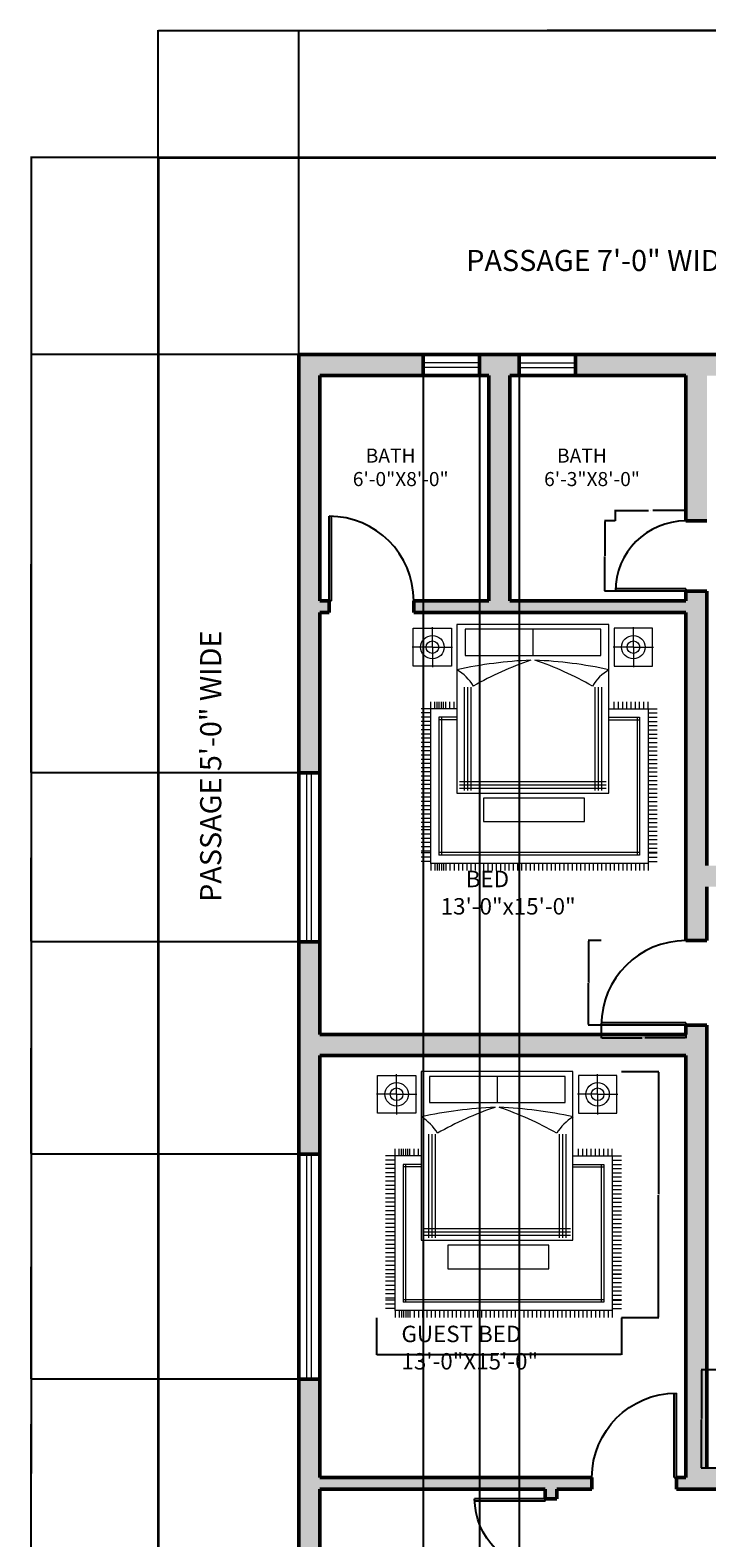
# Model space of a CAD drawing. Units: inches. Extents: x 2447 to 3157, y 2799 to 3988.
# Tile 3 of 9: x 2447 to 2735, y 3345 to 3988. Entities that reach past the tile are written whole.
import ezdxf

# ---------------------------------------------------------------- set-up
doc = ezdxf.new("R2010")
doc.units = ezdxf.units.IN
for name, color, linetype, lineweight in [('A-ANNO-DIMS', 2, 'Continuous', 18), ('A-AREA-IDEN', 7, 'Continuous', 25), ('A-DOOR', 3, 'Continuous', 25), ('A-FURN', 8, 'Continuous', 18), ('A-GLAZ', 4, 'Continuous', 18), ('A-WALL', 7, 'Continuous', 50), ('A-WALL-PATT', 252, 'Continuous', 13), ('C-PROP', 6, 'Continuous', 35)]:
    doc.layers.add(name, color=color, linetype=linetype, lineweight=lineweight)
doc.styles.get("Standard").update_dxf_attribs({"font": 'arial.ttf'})
doc.dimstyles.get("Standard").update_dxf_attribs({"dimtxt": 0.18, "dimasz": 0.18, "dimexe": 0.18, "dimexo": 0.0625, "dimgap": 0.09, "dimtad": 0, "dimtih": 1, "dimtoh": 1, "dimdec": 4, "dimzin": 0, "dimdsep": 46, "dimtxsty": 'Standard', "dimcen": 0.09, "dimadec": 0, "dimazin": 0, "dimtfac": 1, "dimtdec": 4, "dimtofl": 0, "dimtmove": 0, "dimatfit": 3, "dimfxl": 1, "dimtolj": 1, "dimtzin": 0, "dimarcsym": 0})

# ---------------------------------------------------------------- blocks, each defined once
blk = doc.blocks.new('A$C462B680F')
for p, q in [((0.011, 2.874, -0.291), (0.465, 2.874, -0.291)), ((0.011, 2.424, -0.291), (0.011, 2.874, -0.291)), ((0.238, 2.649, -0.561), (0.238, 2.887, -0.561)), ((0.465, 2.874, -0.291), (0.465, 2.424, -0.291)), ((2.33, 2.918, -0.291), (0.53, 2.918, -0.291)), ((0.53, 2.918, -0.291), (0.53, 0.918, -0.291)), ((2.33, 0.918, -0.291), (2.33, 2.918, -0.291)), ((2.849, 2.874, -0.291), (2.395, 2.874, -0.291)), ((2.395, 2.874, -0.291), (2.395, 2.424, -0.291)), ((2.622, 2.649, -0.561), (2.622, 2.887, -0.561)), ((2.849, 2.424, -0.291), (2.849, 2.874, -0.291)), ((1.434, 2.861, -0.291), (0.627, 2.861, -0.291)), ((0.627, 2.861, -0.291), (0.627, 2.55, -0.291)), ((1.43, 2.861, -0.291), (1.43, 2.55, -0.291)), ((2.237, 2.861, -0.291), (1.43, 2.861, -0.291)), ((1.434, 2.55, -0.291), (1.434, 2.861, -0.291)), ((2.237, 2.55, -0.291), (2.237, 2.861, -0.291)), ((0.238, 2.649, -0.561), (0, 2.649, -0.561)), ((0.238, 2.649, -0.561), (0.238, 2.411, -0.561)), ((0.238, 2.649, -0.561), (0.476, 2.649, -0.561)), ((0.627, 2.55, -0.291), (1.434, 2.55, -0.291)), ((1.43, 2.55, -0.291), (2.237, 2.55, -0.291)), ((2.622, 2.649, -0.561), (2.384, 2.649, -0.561)), ((2.622, 2.649, -0.561), (2.622, 2.411, -0.561)), ((2.622, 2.649, -0.561), (2.861, 2.649, -0.561)), ((0.465, 2.424, -0.291), (0.011, 2.424, -0.291)), ((2.395, 2.424, -0.291), (2.849, 2.424, -0.291)), ((0.615, 2.176, -0.291), (0.615, 0.947, -0.291)), ((0.655, 2.176, -0.291), (0.655, 0.947, -0.291)), ((0.695, 2.176, -0.291), (0.695, 0.947, -0.291)), ((2.165, 2.176, -0.291), (2.165, 0.947, -0.291)), ((2.205, 2.176, -0.291), (2.205, 0.947, -0.291)), ((2.245, 2.176, -0.291), (2.245, 0.947, -0.291)), ((0.219, 1.918, -0.291), (0.219, 2, -0.291)), ((0.269, 1.918, -0.291), (0.269, 2, -0.291)), ((0.296, 1.918, -0.291), (0.296, 2, -0.291)), ((0.319, 1.918, -0.291), (0.319, 2, -0.291)), ((0.346, 1.918, -0.291), (0.346, 2, -0.291)), ((0.369, 1.918, -0.291), (0.369, 2, -0.291)), ((0.396, 1.918, -0.291), (0.396, 2, -0.291)), ((0.446, 1.918, -0.291), (0.446, 2, -0.291)), ((0.496, 1.918, -0.291), (0.496, 2, -0.291)), ((2.396, 1.918, -0.291), (2.396, 2, -0.291)), ((2.446, 1.918, -0.291), (2.446, 2, -0.291)), ((2.496, 1.918, -0.291), (2.496, 2, -0.291)), ((2.546, 1.918, -0.291), (2.546, 2, -0.291)), ((2.596, 1.918, -0.291), (2.596, 2, -0.291)), ((2.646, 1.918, -0.291), (2.646, 2, -0.291)), ((2.696, 1.918, -0.291), (2.696, 2, -0.291)), ((2.746, 1.918, -0.291), (2.746, 2, -0.291)), ((2.796, 1.918, -0.291), (2.796, 2, -0.291)), ((0.215, 1.918, -0.291), (0.105, 1.918, -0.291)), ((0.215, 1.868, -0.291), (0.105, 1.868, -0.291)), ((0.215, 1.818, -0.291), (0.105, 1.818, -0.291)), ((0.215, 1.918, -0.291), (0.215, 0.082, -0.291)), ((0.53, 1.918, -0.291), (0.215, 1.918, -0.291)), ((0.315, 1.818, -0.291), (0.315, 0.182, -0.291)), ((0.53, 1.818, -0.291), (0.315, 1.818, -0.291)), ((0.345, 1.818, -0.291), (0.345, 0.182, -0.291)), ((2.33, 1.918, -0.291), (2.796, 1.918, -0.291)), ((2.33, 1.818, -0.291), (2.696, 1.818, -0.291)), ((2.666, 1.818, -0.291), (2.666, 0.182, -0.291)), ((2.696, 1.818, -0.291), (2.696, 0.182, -0.291)), ((2.796, 1.918, -0.291), (2.796, 0.082, -0.291)), ((2.796, 1.918, -0.291), (2.906, 1.918, -0.291)), ((2.796, 1.868, -0.291), (2.906, 1.868, -0.291)), ((2.796, 1.818, -0.291), (2.906, 1.818, -0.291)), ((0.215, 1.768, -0.291), (0.105, 1.768, -0.291)), ((0.215, 1.718, -0.291), (0.105, 1.718, -0.291)), ((0.215, 1.668, -0.291), (0.105, 1.668, -0.291)), ((0.215, 1.618, -0.291), (0.105, 1.618, -0.291)), ((0.53, 1.788, -0.291), (0.315, 1.788, -0.291)), ((2.33, 1.788, -0.291), (2.696, 1.788, -0.291)), ((2.796, 1.768, -0.291), (2.906, 1.768, -0.291)), ((2.796, 1.718, -0.291), (2.906, 1.718, -0.291)), ((2.796, 1.668, -0.291), (2.906, 1.668, -0.291)), ((2.796, 1.618, -0.291), (2.906, 1.618, -0.291)), ((0.215, 1.568, -0.291), (0.105, 1.568, -0.291)), ((0.215, 1.518, -0.291), (0.105, 1.518, -0.291)), ((0.215, 1.468, -0.291), (0.105, 1.468, -0.291)), ((2.796, 1.568, -0.291), (2.906, 1.568, -0.291)), ((2.796, 1.518, -0.291), (2.906, 1.518, -0.291)), ((2.796, 1.468, -0.291), (2.906, 1.468, -0.291)), ((0.215, 1.418, -0.291), (0.105, 1.418, -0.291)), ((0.215, 1.368, -0.291), (0.105, 1.368, -0.291)), ((0.215, 1.318, -0.291), (0.105, 1.318, -0.291)), ((0.215, 1.268, -0.291), (0.105, 1.268, -0.291)), ((2.796, 1.418, -0.291), (2.906, 1.418, -0.291)), ((2.796, 1.368, -0.291), (2.906, 1.368, -0.291)), ((2.796, 1.318, -0.291), (2.906, 1.318, -0.291)), ((2.796, 1.268, -0.291), (2.906, 1.268, -0.291)), ((0.215, 1.218, -0.291), (0.105, 1.218, -0.291)), ((0.215, 1.168, -0.291), (0.105, 1.168, -0.291)), ((0.215, 1.118, -0.291), (0.105, 1.118, -0.291)), ((2.796, 1.218, -0.291), (2.906, 1.218, -0.291)), ((2.796, 1.168, -0.291), (2.906, 1.168, -0.291)), ((2.796, 1.118, -0.291), (2.906, 1.118, -0.291)), ((0.215, 1.068, -0.291), (0.105, 1.068, -0.291)), ((0.215, 1.018, -0.291), (0.105, 1.018, -0.291)), ((0.215, 0.968, -0.291), (0.105, 0.968, -0.291)), ((0.215, 0.918, -0.291), (0.105, 0.918, -0.291)), ((0.53, 0.918, -0.291), (2.33, 0.918, -0.291)), ((0.558, 1.057, -0.291), (2.299, 1.057, -0.291)), ((0.558, 1.017, -0.291), (2.299, 1.017, -0.291)), ((0.558, 0.977, -0.291), (2.299, 0.977, -0.291)), ((2.796, 1.068, -0.291), (2.906, 1.068, -0.291)), ((2.796, 1.018, -0.291), (2.906, 1.018, -0.291)), ((2.796, 0.968, -0.291), (2.906, 0.968, -0.291)), ((2.796, 0.918, -0.291), (2.906, 0.918, -0.291)), ((0.215, 0.868, -0.291), (0.105, 0.868, -0.291)), ((0.215, 0.818, -0.291), (0.105, 0.818, -0.291)), ((0.215, 0.768, -0.291), (0.105, 0.768, -0.291)), ((0.215, 0.718, -0.291), (0.105, 0.718, -0.291)), ((0.844, 0.859, -0.291), (0.844, 0.579, -0.291)), ((2.044, 0.859, -0.291), (0.844, 0.859, -0.291)), ((2.044, 0.579, -0.291), (2.044, 0.859, -0.291)), ((2.796, 0.868, -0.291), (2.906, 0.868, -0.291)), ((2.796, 0.818, -0.291), (2.906, 0.818, -0.291)), ((2.796, 0.768, -0.291), (2.906, 0.768, -0.291)), ((2.796, 0.718, -0.291), (2.906, 0.718, -0.291)), ((0.215, 0.668, -0.291), (0.105, 0.668, -0.291)), ((0.215, 0.618, -0.291), (0.105, 0.618, -0.291)), ((0.215, 0.568, -0.291), (0.105, 0.568, -0.291)), ((0.844, 0.579, -0.291), (2.044, 0.579, -0.291)), ((2.796, 0.668, -0.291), (2.906, 0.668, -0.291)), ((2.796, 0.618, -0.291), (2.906, 0.618, -0.291)), ((2.796, 0.568, -0.291), (2.906, 0.568, -0.291)), ((0.215, 0.518, -0.291), (0.105, 0.518, -0.291)), ((0.215, 0.48, -0.291), (0.105, 0.48, -0.291)), ((0.215, 0.43, -0.291), (0.105, 0.43, -0.291)), ((0.215, 0.38, -0.291), (0.105, 0.38, -0.291)), ((2.796, 0.518, -0.291), (2.906, 0.518, -0.291)), ((2.796, 0.516, -0.291), (2.906, 0.516, -0.291)), ((2.796, 0.466, -0.291), (2.906, 0.466, -0.291)), ((2.796, 0.416, -0.291), (2.906, 0.416, -0.291)), ((2.796, 0.366, -0.291), (2.906, 0.366, -0.291)), ((0.215, 0.33, -0.291), (0.105, 0.33, -0.291)), ((0.215, 0.28, -0.291), (0.105, 0.28, -0.291)), ((0.215, 0.23, -0.291), (0.105, 0.23, -0.291)), ((0.215, 0.207, -0.291), (0.105, 0.207, -0.291)), ((0.215, 0.207, -0.291), (0.105, 0.207, -0.291)), ((2.696, 0.212, -0.291), (0.315, 0.212, -0.291)), ((2.696, 0.182, -0.291), (0.315, 0.182, -0.291)), ((2.796, 0.316, -0.291), (2.906, 0.316, -0.291)), ((2.796, 0.266, -0.291), (2.906, 0.266, -0.291)), ((2.796, 0.216, -0.291), (2.906, 0.216, -0.291)), ((2.796, 0.207, -0.291), (2.906, 0.207, -0.291)), ((2.796, 0.207, -0.291), (2.906, 0.207, -0.291)), ((0.215, 0.157, -0.291), (0.105, 0.157, -0.291)), ((0.215, 0.107, -0.291), (0.105, 0.107, -0.291)), ((2.796, 0.082, -0.291), (0.215, 0.082, -0.291)), ((0.219, 0.082, -0.291), (0.219, 0, -0.291)), ((0.269, 0.082, -0.291), (0.269, 0, -0.291)), ((0.296, 0.082, -0.291), (0.296, 0, -0.291)), ((0.319, 0.082, -0.291), (0.319, 0, -0.291)), ((0.346, 0.082, -0.291), (0.346, 0, -0.291)), ((0.369, 0.082, -0.291), (0.369, 0, -0.291)), ((0.396, 0.082, -0.291), (0.396, 0, -0.291)), ((0.446, 0.082, -0.291), (0.446, 0, -0.291)), ((0.496, 0.082, -0.291), (0.496, 0, -0.291)), ((0.546, 0.082, -0.291), (0.546, 0, -0.291)), ((0.596, 0.082, -0.291), (0.596, 0, -0.291)), ((0.646, 0.082, -0.291), (0.646, 0, -0.291)), ((0.696, 0.082, -0.291), (0.696, 0, -0.291)), ((0.746, 0.082, -0.291), (0.746, 0, -0.291)), ((0.796, 0.082, -0.291), (0.796, 0, -0.291)), ((0.846, 0.082, -0.291), (0.846, 0, -0.291)), ((0.896, 0.082, -0.291), (0.896, 0, -0.291)), ((0.946, 0.082, -0.291), (0.946, 0, -0.291)), ((0.996, 0.082, -0.291), (0.996, 0, -0.291)), ((1.046, 0.082, -0.291), (1.046, 0, -0.291)), ((1.096, 0.082, -0.291), (1.096, 0, -0.291)), ((1.146, 0.082, -0.291), (1.146, 0, -0.291)), ((1.196, 0.082, -0.291), (1.196, 0, -0.291)), ((1.246, 0.082, -0.291), (1.246, 0, -0.291)), ((1.296, 0.082, -0.291), (1.296, 0, -0.291)), ((1.346, 0.082, -0.291), (1.346, 0, -0.291)), ((1.346, 0.082, -0.291), (1.346, 0, -0.291)), ((1.396, 0.082, -0.291), (1.396, 0, -0.291)), ((1.396, 0.082, -0.291), (1.396, 0, -0.291)), ((1.446, 0.082, -0.291), (1.446, 0, -0.291)), ((1.446, 0.082, -0.291), (1.446, 0, -0.291)), ((1.496, 0.082, -0.291), (1.496, 0, -0.291)), ((1.496, 0.082, -0.291), (1.496, 0, -0.291)), ((1.546, 0.082, -0.291), (1.546, 0, -0.291)), ((1.596, 0.082, -0.291), (1.596, 0, -0.291)), ((1.646, 0.082, -0.291), (1.646, 0, -0.291)), ((1.696, 0.082, -0.291), (1.696, 0, -0.291)), ((1.746, 0.082, -0.291), (1.746, 0, -0.291)), ((1.796, 0.082, -0.291), (1.796, 0, -0.291)), ((1.846, 0.082, -0.291), (1.846, 0, -0.291)), ((1.846, 0.082, -0.291), (1.846, 0, -0.291)), ((1.896, 0.082, -0.291), (1.896, 0, -0.291)), ((1.946, 0.082, -0.291), (1.946, 0, -0.291)), ((1.996, 0.082, -0.291), (1.996, 0, -0.291)), ((2.046, 0.082, -0.291), (2.046, 0, -0.291)), ((2.096, 0.082, -0.291), (2.096, 0, -0.291)), ((2.146, 0.082, -0.291), (2.146, 0, -0.291)), ((2.196, 0.082, -0.291), (2.196, 0, -0.291)), ((2.246, 0.082, -0.291), (2.246, 0, -0.291)), ((2.296, 0.082, -0.291), (2.296, 0, -0.291)), ((2.346, 0.082, -0.291), (2.346, 0, -0.291)), ((2.396, 0.082, -0.291), (2.396, 0, -0.291)), ((2.446, 0.082, -0.291), (2.446, 0, -0.291)), ((2.496, 0.082, -0.291), (2.496, 0, -0.291)), ((2.546, 0.082, -0.291), (2.546, 0, -0.291)), ((2.596, 0.082, -0.291), (2.596, 0, -0.291)), ((2.646, 0.082, -0.291), (2.646, 0, -0.291)), ((2.696, 0.082, -0.291), (2.696, 0, -0.291)), ((2.746, 0.082, -0.291), (2.746, 0, -0.291)), ((2.796, 0.157, -0.291), (2.906, 0.157, -0.291)), ((2.796, 0.107, -0.291), (2.906, 0.107, -0.291)), ((2.796, 0.082, -0.291), (2.796, 0, -0.291))]:
    blk.add_line(p, q)
for centre, radius in [((0.238, 2.649, -0.561), 0.139), ((0.238, 2.649, -0.561), 0.075), ((2.622, 2.649, -0.561), 0.139), ((2.622, 2.649, -0.561), 0.075)]:
    blk.add_circle(centre, radius)
for centre, radius, start, end in [((1.618, -2.572, -0.291), 5.071, 92.3872, 102.3913), ((0.231, 1.886, -0.291), 0.578, 31.4118, 58.8491), ((2.601, -1.074, -0.291), 3.763, 108.5127, 119.9306), ((1.243, -2.572, -0.291), 5.071, 77.6087, 87.6128), ((0.259, -1.074, -0.291), 3.763, 60.0694, 71.4873), ((2.63, 1.886, -0.291), 0.578, 121.1509, 148.5882)]:
    blk.add_arc(centre, radius, start, end)
blk = doc.blocks.new('DOOR-SWING-36IN')
for p, q in [((0, 0), (0, 36)), ((1, 0), (1, 35.99)), ((1, 0), (0, 0))]:
    blk.add_line(p, q)
blk.add_arc((0, 0), 36, 0, 90)
blk = doc.blocks.new('DOOR-SWING-30IN')
for p, q in [((0, 1), (-29.98, 1)), ((0, 1), (0, 0)), ((0, 0), (-30, 0))]:
    blk.add_line(p, q)
blk.add_arc((0, 0), 30, 90, 180)
blk = doc.blocks.new('GLAZING-24IN')
for p, q in [((0, 0), (0, 24)), ((2, 0), (2, 24))]:
    blk.add_line(p, q)
blk = doc.blocks.new('*D16')
at = {"layer": 'A-ANNO-DIMS', "color": 0, "lineweight": -2, "transparency": 16777216}
for p, q in [((2690.3, 3599.7), (2684.79, 3599.7)), ((2684.97, 3599.52), (2684.97, 3581.88)), ((2684.97, 3563.88), (2684.97, 3581.52)), ((2690.3, 3563.7), (2684.79, 3563.7))]:
    blk.add_line(p, q, dxfattribs=at)
at = {"layer": 'A-ANNO-DIMS', "color": 0, "transparency": 16777216}
for points in [[(2684.94, 3599.52), (2685, 3599.52), (2684.97, 3599.7)], [(2684.94, 3563.88), (2685, 3563.88), (2684.97, 3563.7)]]:
    blk.add_solid(points, dxfattribs=at)
at = {"layer": 'Defpoints', "color": 0, "transparency": 16777216}
for p in [(2684.97, 3599.7), (2690.37, 3599.7), (2690.37, 3563.7)]:
    blk.add_point(p, dxfattribs=at)
at = {"layer": 'A-ANNO-DIMS', "color": 0, "transparency": 16777216, "insert": (2684.97, 3581.7), "char_height": 0.18, "attachment_point": 5}
blk.add_mtext('\\A1;DOOR 36 TYP.', dxfattribs=at)
blk = doc.blocks.new('*D17')
at = {"layer": 'A-ANNO-DIMS', "color": 0, "lineweight": -2, "transparency": 16777216}
for p, q in [((2690.37, 3563.64), (2690.37, 3558.12)), ((2726.37, 3563.64), (2726.37, 3558.12)), ((2690.55, 3558.3), (2707.84, 3558.3)), ((2726.19, 3558.3), (2708.9, 3558.3))]:
    blk.add_line(p, q, dxfattribs=at)
at = {"layer": 'A-ANNO-DIMS', "color": 0, "transparency": 16777216}
for points in [[(2690.55, 3558.33), (2690.55, 3558.27), (2690.37, 3558.3)], [(2726.19, 3558.33), (2726.19, 3558.27), (2726.37, 3558.3)]]:
    blk.add_solid(points, dxfattribs=at)
at = {"layer": 'Defpoints', "color": 0, "transparency": 16777216}
for p in [(2690.37, 3563.7), (2726.37, 3563.7), (2690.37, 3558.3)]:
    blk.add_point(p, dxfattribs=at)
at = {"layer": 'A-ANNO-DIMS', "color": 0, "transparency": 16777216, "insert": (2708.37, 3558.3), "char_height": 0.18, "attachment_point": 5}
blk.add_mtext('\\A1;36 TYP.', dxfattribs=at)
blk = doc.blocks.new('*D18')
at = {"layer": 'A-ANNO-DIMS', "color": 0, "lineweight": -2, "transparency": 16777216}
for p, q in [((2696.37, 3778.76), (2696.37, 3783.38)), ((2696.55, 3783.2), (2710.43, 3783.2)), ((2726.19, 3783.2), (2712.3, 3783.2)), ((2726.37, 3778.76), (2726.37, 3783.38))]:
    blk.add_line(p, q, dxfattribs=at)
at = {"layer": 'A-ANNO-DIMS', "color": 0, "transparency": 16777216}
for points in [[(2696.55, 3783.23), (2696.55, 3783.17), (2696.37, 3783.2)], [(2726.19, 3783.23), (2726.19, 3783.17), (2726.37, 3783.2)]]:
    blk.add_solid(points, dxfattribs=at)
at = {"layer": 'Defpoints', "color": 0, "transparency": 16777216}
for p in [(2726.37, 3783.2), (2696.37, 3778.7), (2726.37, 3778.7)]:
    blk.add_point(p, dxfattribs=at)
at = {"layer": 'A-ANNO-DIMS', "color": 0, "transparency": 16777216, "insert": (2711.37, 3783.2), "char_height": 0.18, "attachment_point": 5}
blk.add_mtext('\\A1;DOOR 30 TYP.', dxfattribs=at)
blk = doc.blocks.new('*D19')
at = {"layer": 'A-ANNO-DIMS', "color": 0, "lineweight": -2, "transparency": 16777216}
for p, q in [((2696.3, 3778.7), (2691.69, 3778.7)), ((2691.87, 3778.52), (2691.87, 3763.88)), ((2691.87, 3748.88), (2691.87, 3763.52)), ((2696.3, 3748.7), (2691.69, 3748.7))]:
    blk.add_line(p, q, dxfattribs=at)
at = {"layer": 'A-ANNO-DIMS', "color": 0, "transparency": 16777216}
for points in [[(2691.84, 3778.52), (2691.9, 3778.52), (2691.87, 3778.7)], [(2691.84, 3748.88), (2691.9, 3748.88), (2691.87, 3748.7)]]:
    blk.add_solid(points, dxfattribs=at)
at = {"layer": 'Defpoints', "color": 0, "transparency": 16777216}
for p in [(2691.87, 3778.7), (2696.37, 3778.7), (2696.37, 3748.7)]:
    blk.add_point(p, dxfattribs=at)
at = {"layer": 'A-ANNO-DIMS', "color": 0, "transparency": 16777216, "insert": (2691.87, 3763.7), "char_height": 0.18, "attachment_point": 5}
blk.add_mtext('\\A1;30 TYP.', dxfattribs=at)
blk = doc.blocks.new('*D20')
at = {"layer": 'A-ANNO-DIMS', "color": 0, "lineweight": -2, "transparency": 16777216}
for p, q in [((2739.3, 3416.7), (2732.89, 3416.7)), ((2733.07, 3416.52), (2733.07, 3395.88)), ((2733.07, 3374.88), (2733.07, 3395.52)), ((2739.3, 3374.7), (2732.89, 3374.7))]:
    blk.add_line(p, q, dxfattribs=at)
at = {"layer": 'A-ANNO-DIMS', "color": 0, "transparency": 16777216}
for points in [[(2733.04, 3416.52), (2733.1, 3416.52), (2733.07, 3416.7)], [(2733.04, 3374.88), (2733.1, 3374.88), (2733.07, 3374.7)]]:
    blk.add_solid(points, dxfattribs=at)
at = {"layer": 'Defpoints', "color": 0, "transparency": 16777216}
for p in [(2733.07, 3416.7), (2739.37, 3416.7), (2739.37, 3374.7)]:
    blk.add_point(p, dxfattribs=at)
at = {"layer": 'A-ANNO-DIMS', "color": 0, "transparency": 16777216, "insert": (2733.07, 3395.7), "char_height": 0.18, "attachment_point": 5}
blk.add_mtext('\\A1;DOOR 42 TYP.', dxfattribs=at)
blk = doc.blocks.new('*D26')
at = {"layer": 'A-ANNO-DIMS', "color": 0, "lineweight": -2, "transparency": 16777216}
for p, q in [((2699.05, 3543.84), (2714.9, 3543.84)), ((2714.72, 3543.66), (2714.72, 3491.58)), ((2714.72, 3439.13), (2714.72, 3491.21)), ((2699.05, 3438.95), (2714.9, 3438.95))]:
    blk.add_line(p, q, dxfattribs=at)
at = {"layer": 'A-ANNO-DIMS', "color": 0, "transparency": 16777216}
for points in [[(2714.69, 3543.66), (2714.75, 3543.66), (2714.72, 3543.84)], [(2714.69, 3439.13), (2714.75, 3439.13), (2714.72, 3438.95)]]:
    blk.add_solid(points, dxfattribs=at)
at = {"layer": 'Defpoints', "color": 0, "transparency": 16777216}
for p in [(2698.99, 3543.84), (2714.72, 3543.84), (2698.99, 3438.95)]:
    blk.add_point(p, dxfattribs=at)
at = {"layer": 'A-ANNO-DIMS', "color": 0, "transparency": 16777216, "insert": (2714.72, 3491.39), "char_height": 0.18, "attachment_point": 5}
blk.add_mtext('\\A1;BED GROUP 105 TYP.', dxfattribs=at)
blk = doc.blocks.new('*D27')
at = {"layer": 'A-ANNO-DIMS', "color": 0, "lineweight": -2, "transparency": 16777216}
for p, q in [((2594.54, 3438.88), (2594.54, 3423.03)), ((2698.99, 3438.88), (2698.99, 3423.03)), ((2594.72, 3423.21), (2646.18, 3423.21)), ((2698.81, 3423.21), (2647.36, 3423.21))]:
    blk.add_line(p, q, dxfattribs=at)
at = {"layer": 'A-ANNO-DIMS', "color": 0, "transparency": 16777216}
for points in [[(2594.72, 3423.24), (2594.72, 3423.18), (2594.54, 3423.21)], [(2698.81, 3423.24), (2698.81, 3423.18), (2698.99, 3423.21)]]:
    blk.add_solid(points, dxfattribs=at)
at = {"layer": 'Defpoints', "color": 0, "transparency": 16777216}
for p in [(2594.54, 3438.95), (2698.99, 3438.95), (2698.99, 3423.21)]:
    blk.add_point(p, dxfattribs=at)
at = {"layer": 'A-ANNO-DIMS', "color": 0, "transparency": 16777216, "insert": (2646.77, 3423.21), "char_height": 0.18, "attachment_point": 5}
blk.add_mtext('\\A1;104 TYP.', dxfattribs=at)
blk = doc.blocks.new('*D45')
at = {"layer": 'A-ANNO-DIMS', "color": 0, "lineweight": -2, "transparency": 16777216}
for p, q in [((2501.3, 3933.7), (2447.04, 3933.7)), ((2447.22, 3933.52), (2447.22, 3393.88)), ((2447.22, 2853.88), (2447.22, 3393.52)), ((2501.3, 2853.7), (2447.04, 2853.7))]:
    blk.add_line(p, q, dxfattribs=at)
at = {"layer": 'A-ANNO-DIMS', "color": 0, "transparency": 16777216}
for points in [[(2447.19, 3933.52), (2447.25, 3933.52), (2447.22, 3933.7)], [(2447.19, 2853.88), (2447.25, 2853.88), (2447.22, 2853.7)]]:
    blk.add_solid(points, dxfattribs=at)
at = {"layer": 'Defpoints', "color": 0, "transparency": 16777216}
for p in [(2447.22, 3933.7), (2501.37, 3933.7), (2501.37, 2853.7)]:
    blk.add_point(p, dxfattribs=at)
at = {"layer": 'A-ANNO-DIMS', "color": 0, "transparency": 16777216, "insert": (2447.22, 3393.7), "char_height": 0.18, "attachment_point": 5}
blk.add_mtext('\\A1;1080', dxfattribs=at)
blk = doc.blocks.new('*D46')
at = {"layer": 'A-ANNO-DIMS', "color": 0, "lineweight": -2, "transparency": 16777216}
for p, q in [((2561.37, 3849.76), (2561.37, 3988.03)), ((2561.55, 3987.85), (2803.57, 3987.85)), ((3046.19, 3987.85), (2804.16, 3987.85)), ((3046.37, 3825.76), (3046.37, 3988.03))]:
    blk.add_line(p, q, dxfattribs=at)
at = {"layer": 'A-ANNO-DIMS', "color": 0, "transparency": 16777216}
for points in [[(2561.55, 3987.88), (2561.55, 3987.82), (2561.37, 3987.85)], [(3046.19, 3987.88), (3046.19, 3987.82), (3046.37, 3987.85)]]:
    blk.add_solid(points, dxfattribs=at)
at = {"layer": 'Defpoints', "color": 0, "transparency": 16777216}
for p in [(3046.37, 3987.85), (2561.37, 3849.7), (3046.37, 3825.7)]:
    blk.add_point(p, dxfattribs=at)
at = {"layer": 'A-ANNO-DIMS', "color": 0, "transparency": 16777216, "insert": (2803.87, 3987.85), "char_height": 0.18, "attachment_point": 5}
blk.add_mtext('\\A1;485', dxfattribs=at)
blk = doc.blocks.new('*D52')
at = {"layer": 'A-ANNO-DIMS', "color": 0, "lineweight": -2, "transparency": 16777216}
for p, q in [((2501.37, 3933.76), (2501.37, 3988.03)), ((2501.55, 3987.85), (2666.54, 3987.85)), ((2832.28, 3987.85), (2667.29, 3987.85)), ((2832.46, 3933.76), (2832.46, 3988.03))]:
    blk.add_line(p, q, dxfattribs=at)
at = {"layer": 'A-ANNO-DIMS', "color": 0, "transparency": 16777216}
for points in [[(2501.55, 3987.88), (2501.55, 3987.82), (2501.37, 3987.85)], [(2832.28, 3987.88), (2832.28, 3987.82), (2832.46, 3987.85)]]:
    blk.add_solid(points, dxfattribs=at)
at = {"layer": 'Defpoints', "color": 0, "transparency": 16777216}
for p in [(2832.46, 3987.85), (2501.37, 3933.7), (2832.46, 3933.7)]:
    blk.add_point(p, dxfattribs=at)
at = {"layer": 'A-ANNO-DIMS', "color": 0, "transparency": 16777216, "insert": (2666.91, 3987.85), "char_height": 0.18, "attachment_point": 5}
blk.add_mtext('\\A1;331.1', dxfattribs=at)
blk = doc.blocks.new('*D57')
at = {"layer": 'A-ANNO-DIMS', "color": 0, "lineweight": -2, "transparency": 16777216}
for p, q in [((2561.3, 3412.7), (2447.04, 3412.7)), ((2447.22, 3412.52), (2447.22, 3372.5)), ((2447.22, 3332.11), (2447.22, 3372.13)), ((2561.3, 3331.93), (2447.04, 3331.93))]:
    blk.add_line(p, q, dxfattribs=at)
at = {"layer": 'A-ANNO-DIMS', "color": 0, "transparency": 16777216}
for points in [[(2447.19, 3412.52), (2447.25, 3412.52), (2447.22, 3412.7)], [(2447.19, 3332.11), (2447.25, 3332.11), (2447.22, 3331.93)]]:
    blk.add_solid(points, dxfattribs=at)
at = {"layer": 'Defpoints', "color": 0, "transparency": 16777216}
for p in [(2447.22, 3412.7), (2561.37, 3412.7), (2561.37, 3331.93)]:
    blk.add_point(p, dxfattribs=at)
at = {"layer": 'A-ANNO-DIMS', "color": 0, "transparency": 16777216, "insert": (2447.22, 3372.31), "char_height": 0.18, "attachment_point": 5}
blk.add_mtext('\\A1;80.77', dxfattribs=at)
blk = doc.blocks.new('*D58')
at = {"layer": 'A-ANNO-DIMS', "color": 0, "lineweight": -2, "transparency": 16777216}
for p, q in [((2561.3, 3508.7), (2447.04, 3508.7)), ((2447.22, 3508.52), (2447.22, 3460.88)), ((2447.22, 3412.88), (2447.22, 3460.52)), ((2561.3, 3412.7), (2447.04, 3412.7))]:
    blk.add_line(p, q, dxfattribs=at)
at = {"layer": 'A-ANNO-DIMS', "color": 0, "transparency": 16777216}
for points in [[(2447.19, 3508.52), (2447.25, 3508.52), (2447.22, 3508.7)], [(2447.19, 3412.88), (2447.25, 3412.88), (2447.22, 3412.7)]]:
    blk.add_solid(points, dxfattribs=at)
at = {"layer": 'Defpoints', "color": 0, "transparency": 16777216}
for p in [(2447.22, 3508.7), (2561.37, 3508.7), (2561.37, 3412.7)]:
    blk.add_point(p, dxfattribs=at)
at = {"layer": 'A-ANNO-DIMS', "color": 0, "transparency": 16777216, "insert": (2447.22, 3460.7), "char_height": 0.18, "attachment_point": 5}
blk.add_mtext('\\A1;96', dxfattribs=at)
blk = doc.blocks.new('*D59')
at = {"layer": 'A-ANNO-DIMS', "color": 0, "lineweight": -2, "transparency": 16777216}
for p, q in [((2561.3, 3599.25), (2447.04, 3599.25)), ((2447.22, 3599.07), (2447.22, 3554.16)), ((2447.22, 3508.88), (2447.22, 3553.79)), ((2561.3, 3508.7), (2447.04, 3508.7))]:
    blk.add_line(p, q, dxfattribs=at)
at = {"layer": 'A-ANNO-DIMS', "color": 0, "transparency": 16777216}
for points in [[(2447.19, 3599.07), (2447.25, 3599.07), (2447.22, 3599.25)], [(2447.19, 3508.88), (2447.25, 3508.88), (2447.22, 3508.7)]]:
    blk.add_solid(points, dxfattribs=at)
at = {"layer": 'Defpoints', "color": 0, "transparency": 16777216}
for p in [(2447.22, 3599.25), (2561.37, 3599.25), (2561.37, 3508.7)]:
    blk.add_point(p, dxfattribs=at)
at = {"layer": 'A-ANNO-DIMS', "color": 0, "transparency": 16777216, "insert": (2447.22, 3553.97), "char_height": 0.18, "attachment_point": 5}
blk.add_mtext('\\A1;90.55', dxfattribs=at)
blk = doc.blocks.new('*D60')
at = {"layer": 'A-ANNO-DIMS', "color": 0, "lineweight": -2, "transparency": 16777216}
for p, q in [((2561.3, 3671.25), (2447.04, 3671.25)), ((2447.22, 3671.07), (2447.22, 3635.43)), ((2447.22, 3599.43), (2447.22, 3635.07)), ((2561.3, 3599.25), (2447.04, 3599.25))]:
    blk.add_line(p, q, dxfattribs=at)
at = {"layer": 'A-ANNO-DIMS', "color": 0, "transparency": 16777216}
for points in [[(2447.19, 3671.07), (2447.25, 3671.07), (2447.22, 3671.25)], [(2447.19, 3599.43), (2447.25, 3599.43), (2447.22, 3599.25)]]:
    blk.add_solid(points, dxfattribs=at)
at = {"layer": 'Defpoints', "color": 0, "transparency": 16777216}
for p in [(2447.22, 3671.25), (2561.37, 3671.25), (2561.37, 3599.25)]:
    blk.add_point(p, dxfattribs=at)
at = {"layer": 'A-ANNO-DIMS', "color": 0, "transparency": 16777216, "insert": (2447.22, 3635.25), "char_height": 0.18, "attachment_point": 5}
blk.add_mtext('\\A1;72', dxfattribs=at)
blk = doc.blocks.new('*D61')
at = {"layer": 'A-ANNO-DIMS', "color": 0, "lineweight": -2, "transparency": 16777216}
for p, q in [((2561.3, 3849.7), (2447.04, 3849.7)), ((2447.22, 3849.52), (2447.22, 3760.66)), ((2447.22, 3671.43), (2447.22, 3760.29)), ((2561.3, 3671.25), (2447.04, 3671.25))]:
    blk.add_line(p, q, dxfattribs=at)
at = {"layer": 'A-ANNO-DIMS', "color": 0, "transparency": 16777216}
for points in [[(2447.19, 3849.52), (2447.25, 3849.52), (2447.22, 3849.7)], [(2447.19, 3671.43), (2447.25, 3671.43), (2447.22, 3671.25)]]:
    blk.add_solid(points, dxfattribs=at)
at = {"layer": 'Defpoints', "color": 0, "transparency": 16777216}
for p in [(2447.22, 3849.7), (2561.37, 3849.7), (2561.37, 3671.25)]:
    blk.add_point(p, dxfattribs=at)
at = {"layer": 'A-ANNO-DIMS', "color": 0, "transparency": 16777216, "insert": (2447.22, 3760.47), "char_height": 0.18, "attachment_point": 5}
blk.add_mtext('\\A1;178.45', dxfattribs=at)
blk = doc.blocks.new('*D68')
at = {"layer": 'A-ANNO-DIMS', "color": 0, "lineweight": -2, "transparency": 16777216}
for p, q in [((2561.37, 3849.64), (2561.37, 2799.37)), ((2614.37, 3840.64), (2614.37, 2799.37)), ((2561.55, 2799.55), (2587.65, 2799.55)), ((2614.19, 2799.55), (2588.09, 2799.55))]:
    blk.add_line(p, q, dxfattribs=at)
at = {"layer": 'A-ANNO-DIMS', "color": 0, "transparency": 16777216}
for points in [[(2561.55, 2799.58), (2561.55, 2799.52), (2561.37, 2799.55)], [(2614.19, 2799.58), (2614.19, 2799.52), (2614.37, 2799.55)]]:
    blk.add_solid(points, dxfattribs=at)
at = {"layer": 'Defpoints', "color": 0, "transparency": 16777216}
for p in [(2561.37, 3849.7), (2614.37, 3840.7), (2614.37, 2799.55)]:
    blk.add_point(p, dxfattribs=at)
at = {"layer": 'A-ANNO-DIMS', "color": 0, "transparency": 16777216, "insert": (2587.87, 2799.55), "char_height": 0.18, "attachment_point": 5}
blk.add_mtext('\\A1;53', dxfattribs=at)
blk = doc.blocks.new('*D69')
at = {"layer": 'A-ANNO-DIMS', "color": 0, "lineweight": -2, "transparency": 16777216}
for p, q in [((2638.37, 3840.64), (2638.37, 2799.37)), ((2655.37, 3840.64), (2655.37, 2799.37)), ((2638.55, 2799.55), (2646.66, 2799.55)), ((2655.19, 2799.55), (2647.08, 2799.55))]:
    blk.add_line(p, q, dxfattribs=at)
at = {"layer": 'A-ANNO-DIMS', "color": 0, "transparency": 16777216}
for points in [[(2638.55, 2799.58), (2638.55, 2799.52), (2638.37, 2799.55)], [(2655.19, 2799.58), (2655.19, 2799.52), (2655.37, 2799.55)]]:
    blk.add_solid(points, dxfattribs=at)
at = {"layer": 'Defpoints', "color": 0, "transparency": 16777216}
for p in [(2638.37, 3840.7), (2655.37, 3840.7), (2655.37, 2799.55)]:
    blk.add_point(p, dxfattribs=at)
at = {"layer": 'A-ANNO-DIMS', "color": 0, "transparency": 16777216, "insert": (2646.87, 2799.55), "char_height": 0.18, "attachment_point": 5}
blk.add_mtext('\\A1;17', dxfattribs=at)

msp = doc.modelspace()

# ---------------------------------------------------------------- hatches: boundary and pattern name
at = {"layer": 'A-WALL-PATT'}
h = msp.add_hatch(color=256, dxfattribs=at)
h.dxf.hatch_style = 1
h.paths.add_polyline_path([(2570.3672, 3550.7002), (2726.3672, 3550.7002), (2726.3672, 3370.7002), (2722.3672, 3370.7002), (2722.3672, 3365.7002), (2739.3672, 3365.7002), (2739.3672, 3374.7002), (2735.3672, 3374.7002), (2735.3672, 3563.7002), (2726.3672, 3563.7002), (2726.3672, 3559.7002), (2570.3672, 3559.7002), (2570.3672, 3599.2479), (2561.3672, 3599.2479), (2561.3672, 3508.7002), (2570.3672, 3508.7002)])
h.paths.add_polyline_path([(2570.3672, 3412.7002), (2561.3672, 3412.7002), (2561.3672, 3331.9279), (2570.3672, 3331.9279), (2570.3672, 3365.7002), (2666.3672, 3365.7002), (2666.3672, 3361.7002), (2671.3672, 3361.7002), (2671.3672, 3365.7002), (2686.3672, 3365.7002), (2686.3672, 3370.7002), (2570.3672, 3370.7002)])
h.paths.add_polyline_path([(2965.3672, 3430.7002), (2961.3672, 3430.7002), (2961.3672, 3434.7002), (2952.3672, 3434.7002), (2952.3672, 3430.7002), (2847.6393, 3430.7002), (2812.3672, 3395.4282), (2812.3672, 3374.7002), (2781.3672, 3374.7002), (2781.3672, 3365.7002), (2812.3672, 3365.7002), (2812.3672, 3347.7002), (2821.3672, 3347.7002), (2821.3672, 3391.7002), (2851.3672, 3421.7002), (2965.3672, 3421.7002)])
h.paths.add_polyline_path([(3046.3672, 3430.7002), (3033.3672, 3430.7002), (3033.3672, 3421.7002), (3037.3672, 3421.7002), (3037.3672, 3133.7002), (2971.1661, 3133.7002), (2971.1661, 3124.7002), (3046.3672, 3124.7002)])
h.paths.add_polyline_path([(3046.3672, 3825.7002), (3005.5801, 3825.7002), (3005.5801, 3816.7002), (3037.3672, 3816.7002), (3037.3672, 3655.7002), (2940.3672, 3655.7002), (2940.3672, 3646.7002), (3037.3672, 3646.7002), (3037.3672, 3514.7002), (3033.3672, 3514.7002), (3033.3672, 3505.7002), (3046.3672, 3505.7002)])
h.paths.add_polyline_path([(2821.3672, 3258.7002), (2812.3672, 3258.7002), (2812.3672, 3240.7002), (2808.3672, 3240.7002), (2808.3672, 3231.7002), (2812.3672, 3231.7002), (2812.3672, 3223.0688), (2821.3672, 3223.0688)])
h.paths.add_polyline_path([(2766.3672, 3240.7002), (2707.3672, 3240.7002), (2707.3672, 3234.4466, -1), (2570.3672, 3234.4466), (2570.3672, 3240.5271), (2561.3672, 3240.5271), (2561.3672, 3234.4466, 0.98243292), (2716.3185, 3231.7002), (2766.3672, 3231.7002)])
h.paths.add_polyline_path([(2570.3672, 3307.9279), (2561.3672, 3307.9279), (2561.3672, 3281.7773), (2570.3672, 3281.7773), (2570.3672, 3284.7002), (2671.3672, 3284.7002), (2671.3672, 3331.7002), (2666.3672, 3331.7002), (2666.3672, 3293.7002), (2570.3672, 3293.7002)])
h.paths.add_polyline_path([(2570.3672, 3739.7002), (2574.3672, 3739.7002), (2574.3672, 3744.7002), (2570.3672, 3744.7002), (2570.3672, 3840.7002), (2614.3672, 3840.7002), (2614.3672, 3849.7002), (2561.3672, 3849.7002), (2561.3672, 3671.2479), (2570.3672, 3671.2479)])
h.paths.add_polyline_path([(2735.3672, 3840.7002), (2789.3672, 3840.7002), (2789.3672, 3816.7002), (2798.3672, 3816.7002), (2798.3672, 3849.7002), (2679.3672, 3849.7002), (2679.3672, 3840.7002), (2726.3672, 3840.7002), (2726.3672, 3778.7002), (2735.3672, 3778.7002)])
h.paths.add_polyline_path([(2651.3672, 3840.7002), (2655.3672, 3840.7002), (2655.3672, 3849.7002), (2638.3672, 3849.7002), (2638.3672, 3840.7002), (2642.3672, 3840.7002), (2642.3672, 3744.7002), (2610.3672, 3744.7002), (2610.3672, 3739.7002), (2726.3672, 3739.7002), (2726.3672, 3599.7002), (2735.3672, 3599.7002), (2735.3672, 3622.7002), (2739.3672, 3622.7002), (2739.3672, 3631.7002), (2735.3672, 3631.7002), (2735.3672, 3748.7002), (2726.3672, 3748.7002), (2726.3672, 3744.7002), (2651.3672, 3744.7002)])
h.paths.add_polyline_path([(2900.3672, 3816.7002), (2904.3672, 3816.7002), (2904.3672, 3825.7002), (2882.3672, 3825.7002), (2882.3672, 3816.7002), (2891.3672, 3816.7002), (2891.3672, 3650.4282), (2872.6393, 3631.7002), (2775.3672, 3631.7002), (2775.3672, 3622.7002), (2876.3672, 3622.7002), (2900.3672, 3646.7002), (2904.3672, 3646.7002), (2904.3672, 3655.7002), (2900.3672, 3655.7002)])
h.paths.add_polyline_path([(2957.5801, 3825.7002), (2940.3672, 3825.7002), (2940.3672, 3816.7002), (2957.5801, 3816.7002)], flags=17)

# ---------------------------------------------------------------- linework, layer by layer
at = {"layer": 'A-GLAZ'}
for p, q in [((2564.8672, 3599.2479), (2564.8672, 3671.2479)), ((2566.8672, 3599.2479), (2566.8672, 3671.2479)), ((2564.8672, 3412.7002), (2564.8672, 3508.7002)), ((2566.8672, 3412.7002), (2566.8672, 3508.7002))]:
    msp.add_line(p, q, dxfattribs=at)
at = {"layer": 'A-WALL'}
for p, q in [((2561.3672, 3849.7002), (2561.3672, 3234.4466)), ((2561.3672, 3849.7002), (2798.3672, 3849.7002)), ((2614.3672, 3849.7002), (2614.3672, 3840.7002)), ((2638.3672, 3849.7002), (2638.3672, 3840.7002)), ((2655.3672, 3849.7002), (2655.3672, 3840.7002)), ((2679.3672, 3849.7002), (2679.3672, 3840.7002)), ((2570.3672, 3840.7002), (2642.3672, 3840.7002)), ((2570.3672, 3840.7002), (2570.3672, 3744.7002)), ((2642.3672, 3840.7002), (2642.3672, 3744.7002)), ((2651.3672, 3840.7002), (2651.3672, 3744.7002)), ((2651.3672, 3840.7002), (2726.3672, 3840.7002)), ((2726.3672, 3840.7002), (2726.3672, 3778.7002)), ((2726.3672, 3778.7002), (2735.3672, 3778.7002)), ((2570.3672, 3744.7002), (2574.3672, 3744.7002)), ((2574.3672, 3744.7002), (2574.3672, 3739.7002)), ((2610.3672, 3744.7002), (2610.3672, 3739.7002)), ((2610.3672, 3744.7002), (2642.3672, 3744.7002)), ((2651.3672, 3744.7002), (2726.3672, 3744.7002)), ((2726.3672, 3748.7002), (2735.3672, 3748.7002)), ((2726.3672, 3748.7002), (2726.3672, 3744.7002)), ((2735.3672, 3748.7002), (2735.3672, 3631.7002)), ((2570.3672, 3739.7002), (2574.3672, 3739.7002)), ((2570.3672, 3739.7002), (2570.3672, 3559.7002)), ((2610.3672, 3739.7002), (2726.3672, 3739.7002)), ((2726.3672, 3739.7002), (2726.3672, 3599.7002)), ((2570.3672, 3671.2479), (2561.3672, 3671.2479)), ((2735.3672, 3622.7002), (2735.3672, 3599.7002)), ((2570.3672, 3599.2479), (2561.3672, 3599.2479)), ((2726.3672, 3599.7002), (2735.3672, 3599.7002)), ((2726.3672, 3563.7002), (2735.3672, 3563.7002)), ((2726.3672, 3559.7002), (2726.3672, 3563.7002)), ((2735.3672, 3563.7002), (2735.3672, 3374.7002)), ((2570.3672, 3559.7002), (2726.3672, 3559.7002)), ((2570.3672, 3550.7002), (2726.3672, 3550.7002)), ((2570.3672, 3550.7002), (2570.3672, 3370.7002)), ((2726.3672, 3550.7002), (2726.3672, 3370.7002)), ((2570.3672, 3508.7002), (2561.3672, 3508.7002)), ((2570.3672, 3412.7002), (2561.3672, 3412.7002)), ((2570.3672, 3370.7002), (2686.3672, 3370.7002)), ((2686.3672, 3370.7002), (2686.3672, 3365.7002)), ((2722.3672, 3370.7002), (2722.3672, 3365.7002)), ((2722.3672, 3370.7002), (2726.3672, 3370.7002)), ((2570.3672, 3365.7002), (2666.3672, 3365.7002)), ((2570.3672, 3365.7002), (2570.3672, 3293.7002)), ((2666.3672, 3365.7002), (2666.3672, 3361.7002)), ((2671.3672, 3365.7002), (2671.3672, 3361.7002)), ((2671.3672, 3365.7002), (2686.3672, 3365.7002)), ((2722.3672, 3365.7002), (2739.3672, 3365.7002)), ((2666.3672, 3361.7002), (2671.3672, 3361.7002))]:
    msp.add_line(p, q, dxfattribs=at)
at = {"layer": 'C-PROP'}
for q in [(3102.3672, 3933.7002), (2501.3672, 2853.7002)]:
    msp.add_line((2501.3672, 3933.7002), q, dxfattribs=at)

# ---------------------------------------------------------------- block references
at = {"layer": 'A-DOOR'}
for name, p in [('DOOR-SWING-36IN', (2574.3672, 3744.7002)), ('DOOR-SWING-30IN', (2726.3672, 3748.7002))]:
    msp.add_blockref(name, p, dxfattribs=at)
at = {"layer": 'A-DOOR', "rotation": 90.00000000000486}
msp.add_blockref('DOOR-SWING-36IN', (2726.3672, 3563.7002), dxfattribs=at)
at = {"layer": 'A-DOOR', "extrusion": (0, 0, -1), "zscale": -1}
msp.add_blockref('DOOR-SWING-36IN', (-2722.3672, 3370.7002), dxfattribs=at)
at = {"layer": 'A-DOOR', "extrusion": (0, 0, -1), "zscale": -1, "rotation": 180}
msp.add_blockref('DOOR-SWING-30IN', (-2666.3672, 3361.7002), dxfattribs=at)
at = {"layer": 'A-FURN', "xscale": 35.94635118840503, "yscale": 35.94635118840503, "zscale": 35.94635118840503}
for p in [(2609.7877, 3629.6508), (2594.5444, 3438.9467)]:
    msp.add_blockref('A$C462B680F', p, dxfattribs=at)
at = {"layer": 'A-GLAZ'}
for p, rotation in [((2638.3672, 3844.2002), 89.99999999999568), ((2655.3672, 3846.2002), 270.0000000000043)]:
    msp.add_blockref('GLAZING-24IN', p, dxfattribs=dict(at, rotation=rotation))

# ---------------------------------------------------------------- texts
at = {"layer": 'A-AREA-IDEN', "attachment_point": 1}
for s, width, insert, char_height in [('PASSAGE 7\'-0" WIDE', 130.290701, (2632.7819, 3894.2968), 9), ('   BATH\\P6\'-0"X8\'-0"', 44.105841, (2584.4112, 3809.5722), 6), ('   BATH\\P6\'-3"X8\'-0"', 44.105841, (2665.9829, 3809.5722), 6), ('              {\\H2.8x;BED\\P13\'-0"x15\'-0"}', 54.088043, (2621.8876, 3629.5056), 2.5), ('GUEST BED\\P13\'-0"X15\'-0"', 88.110154, (2605.1569, 3435.4642), 7)]:
    msp.add_mtext_dynamic_manual_height_columns(s, width=width, gutter_width=12.5, heights=[0], dxfattribs=dict(at, insert=insert, char_height=char_height))
at = {"layer": 'A-AREA-IDEN', "insert": (2519.3177, 3616.2339), "char_height": 9, "attachment_point": 1, "rotation": 90}
msp.add_mtext_dynamic_manual_height_columns('PASSAGE 5\'-0" WIDE', width=130.290701, gutter_width=12.5, heights=[0], dxfattribs=at)

# ---------------------------------------------------------------- dimensions: what is measured, and where the dimension line sits
at = {"layer": 'A-ANNO-DIMS'}
for base, p1, p2, override, picture, middle in [((2832.456, 3987.8502), (2501.3672, 3933.7002), (2832.456, 3933.7002), {"dimdec": 1, "dimlfac": 1, "dimrnd": 0, "dimzin": 0, "dimdsep": 46, "dimlunit": 2}, '*D52', (2666.9116, 3987.8502)), ((3046.3672, 3987.8502), (2561.3672, 3849.7002), (3046.3672, 3825.7002), {"dimdec": 0, "dimlfac": 1, "dimrnd": 0, "dimzin": 0, "dimdsep": 46, "dimlunit": 2}, '*D46', (2803.8672, 3987.8502)), ((2614.3672, 2799.5502), (2561.3672, 3849.7002), (2614.3672, 3840.7002), {"dimdec": 0, "dimlfac": 1, "dimrnd": 0, "dimzin": 0, "dimdsep": 46, "dimlunit": 2}, '*D68', (2587.8672, 2799.5502)), ((2655.3672, 2799.5502), (2638.3672, 3840.7002), (2655.3672, 3840.7002), {"dimdec": 0, "dimlfac": 1, "dimrnd": 0, "dimzin": 0, "dimdsep": 46, "dimlunit": 2}, '*D69', (2646.8672, 2799.5502))]:
    dim = msp.add_linear_dim(base=base, p1=p1, p2=p2, dimstyle='Standard', override=override, dxfattribs=at)
    dim.commit()
    dim.dimension.update_dxf_attribs({"geometry": picture, "text_midpoint": middle})
for base, p1, p2, override, picture, middle in [((2447.2172, 3933.7002), (2501.3672, 2853.7002), (2501.3672, 3933.7002), {"dimdec": 0, "dimlfac": 1, "dimrnd": 0, "dimzin": 0, "dimdsep": 46, "dimlunit": 2}, '*D45', (2447.2172, 3393.7002)), ((2447.2172, 3849.7002), (2561.3672, 3671.2479), (2561.3672, 3849.7002), {"dimdec": 2, "dimlfac": 1, "dimrnd": 0, "dimzin": 0, "dimdsep": 46, "dimlunit": 2}, '*D61', (2447.2172, 3760.4741)), ((2447.2172, 3671.2479), (2561.3672, 3599.2479), (2561.3672, 3671.2479), {"dimdec": 0, "dimlfac": 1, "dimrnd": 0, "dimzin": 0, "dimdsep": 46, "dimlunit": 2}, '*D60', (2447.2172, 3635.2479)), ((2447.2172, 3599.2479), (2561.3672, 3508.7002), (2561.3672, 3599.2479), {"dimdec": 2, "dimlfac": 1, "dimrnd": 0, "dimzin": 0, "dimdsep": 46, "dimlunit": 2}, '*D59', (2447.2172, 3553.9741)), ((2447.2172, 3508.7002), (2561.3672, 3412.7002), (2561.3672, 3508.7002), {"dimdec": 0, "dimlfac": 1, "dimrnd": 0, "dimzin": 0, "dimdsep": 46, "dimlunit": 2}, '*D58', (2447.2172, 3460.7002)), ((2447.2172, 3412.7002), (2561.3672, 3331.9279), (2561.3672, 3412.7002), {"dimdec": 2, "dimlfac": 1, "dimrnd": 0, "dimzin": 0, "dimdsep": 46, "dimlunit": 2}, '*D57', (2447.2172, 3372.3141))]:
    dim = msp.add_linear_dim(base=base, p1=p1, p2=p2, angle=90, dimstyle='Standard', override=override, dxfattribs=at)
    dim.commit()
    dim.dimension.update_dxf_attribs({"geometry": picture, "text_midpoint": middle})
for base, p1, p2, text, picture, middle in [((2726.3672, 3783.2002), (2696.3672, 3778.7002), (2726.3672, 3778.7002), 'DOOR <> TYP.', '*D18', (2711.3672, 3783.2002)), ((2698.9866, 3423.213), (2594.5444, 3438.9467), (2698.9866, 3438.9467), '<> TYP.', '*D27', (2646.7655, 3423.213))]:
    dim = msp.add_linear_dim(base=base, p1=p1, p2=p2, text=text, dimstyle='Standard', override={"dimdec": 0, "dimlfac": 1, "dimrnd": 0, "dimzin": 0, "dimdsep": 46, "dimlunit": 2}, dxfattribs=at)
    dim.commit()
    dim.dimension.update_dxf_attribs({"geometry": picture, "text_midpoint": middle})
for base, p1, p2, angle, text, picture, middle in [((2691.8672, 3778.7002), (2696.3672, 3748.7002), (2696.3672, 3778.7002), 90, '<> TYP.', '*D19', (2691.8672, 3763.7002)), ((2684.9672, 3599.7002), (2690.3672, 3563.7002), (2690.3672, 3599.7002), 90, 'DOOR <> TYP.', '*D16', (2684.9672, 3581.7002)), ((2690.3672, 3558.3002), (2726.3672, 3563.7002), (2690.3672, 3563.7002), 180, '<> TYP.', '*D17', (2708.3672, 3558.3002)), ((2714.7203, 3543.8383), (2698.9866, 3438.9467), (2698.9866, 3543.8383), 90, 'BED GROUP <> TYP.', '*D26', (2714.7203, 3491.3925)), ((2733.0672, 3416.7002), (2739.3672, 3374.7002), (2739.3672, 3416.7002), 90, 'DOOR <> TYP.', '*D20', (2733.0672, 3395.7002))]:
    dim = msp.add_linear_dim(base=base, p1=p1, p2=p2, angle=angle, text=text, dimstyle='Standard', override={"dimdec": 0, "dimlfac": 1, "dimrnd": 0, "dimzin": 0, "dimdsep": 46, "dimlunit": 2}, dxfattribs=at)
    dim.commit()
    dim.dimension.update_dxf_attribs({"geometry": picture, "text_midpoint": middle})

doc.saveas('drawing.dxf')
